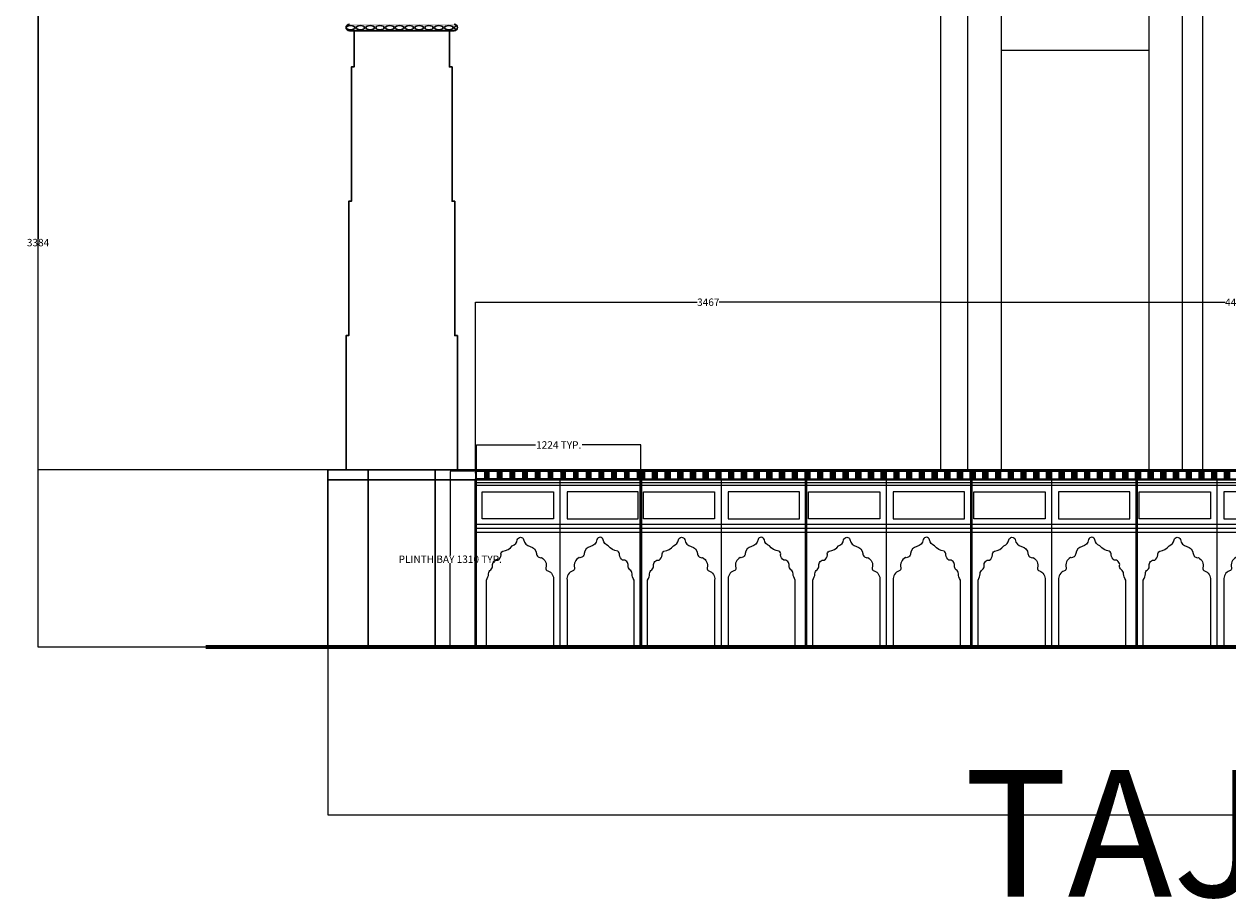
# Model space of a CAD drawing. Units: millimetres. Extents: x 8570 to 49085, y 3782 to 24863.
# Tile 1 of 15: x 8580 to 17549, y 4026 to 10542. Entities that reach past the tile are written whole.
import ezdxf

# ---------------------------------------------------------------- set-up
doc = ezdxf.new("R2010")
doc.units = ezdxf.units.MM
doc.header["$MEASUREMENT"] = 0
doc.header["$PDMODE"] = 3
for name, color, linetype, lineweight in [('A-ANNO-DIMS', 2, 'Continuous', 18), ('A-ANNO-TEXT', 7, 'Continuous', 25), ('A-ELEV-ARCH', 7, 'Continuous', 25), ('A-ELEV-GRND', 7, 'Continuous', 35), ('A-ELEV-MNRT', 7, 'Continuous', 30), ('A-ELEV-PATT', 252, 'Continuous', 13), ('A-ELEV-PIER', 7, 'Continuous', 25), ('A-ELEV-PLIN', 7, 'Continuous', 25)]:
    doc.layers.add(name, color=color, linetype=linetype, lineweight=lineweight)
doc.styles.get("Standard").update_dxf_attribs({"font": 'arial.ttf'})
doc.dimstyles.get("Standard").update_dxf_attribs({"dimtxt": 55, "dimasz": 0.18, "dimexe": 0.18, "dimexo": 0.0625, "dimgap": 0.09, "dimtad": 0, "dimtih": 1, "dimtoh": 1, "dimdec": 0, "dimzin": 0, "dimdsep": 46, "dimtxsty": 'Standard', "dimcen": 0.09, "dimadec": 0, "dimazin": 0, "dimtfac": 1, "dimtdec": 0, "dimtofl": 0, "dimtmove": 0, "dimatfit": 3, "dimfxl": 1, "dimtolj": 1, "dimtzin": 0, "dimarcsym": 0})

# ---------------------------------------------------------------- blocks, each defined once
blk = doc.blocks.new('MINARET-ELEV')
h = blk.add_hatch(color=256)
h.dxf.hatch_style = 1
edge = h.paths.add_edge_path()
edge.add_arc((940, 4615.3), 25, 270, 450, ccw=False)
edge.add_line((940, 4590.3), (160, 4590.3))
edge.add_arc((160, 4615.3), 25, 217.6761, 270, ccw=False)
edge.add_ellipse((127.2, 4613.7), major_axis=(31.8, 0), ratio=0.472441, start_angle=313.43175, end_angle=411.74889)
edge.add_arc((160, 4615.3), 25, 450, 510.08055, ccw=False)
edge.add_line((160, 4640.3), (940, 4640.3))
edge = h.paths.add_edge_path(flags=16)
edge.add_ellipse((347.2, 4613.7), major_axis=(31.8, 0), ratio=0.472441, start_angle=0, end_angle=360, ccw=False)
edge = h.paths.add_edge_path(flags=16)
edge.add_ellipse((420.2, 4613.7), major_axis=(31.8, 0), ratio=0.472441, start_angle=0, end_angle=360, ccw=False)
edge = h.paths.add_edge_path(flags=16)
edge.add_ellipse((274.2, 4613.7), major_axis=(31.8, 0), ratio=0.472441, start_angle=0, end_angle=360, ccw=False)
edge = h.paths.add_edge_path(flags=16)
edge.add_ellipse((493.2, 4613.7), major_axis=(31.8, 0), ratio=0.472441, start_angle=0, end_angle=360, ccw=False)
edge = h.paths.add_edge_path(flags=16)
edge.add_ellipse((198.8, 4613.7), major_axis=(31.8, 0), ratio=0.472441, start_angle=0, end_angle=360, ccw=False)
edge = h.paths.add_edge_path(flags=16)
edge.add_ellipse((566.2, 4613.7), major_axis=(31.8, 0), ratio=0.472441, start_angle=0, end_angle=360, ccw=False)
edge = h.paths.add_edge_path(flags=16)
edge.add_ellipse((639.2, 4613.7), major_axis=(31.8, 0), ratio=0.472441, start_angle=0, end_angle=360, ccw=False)
edge = h.paths.add_edge_path(flags=16)
edge.add_ellipse((712.2, 4613.7), major_axis=(31.8, 0), ratio=0.472441, start_angle=0, end_angle=360, ccw=False)
edge = h.paths.add_edge_path(flags=16)
edge.add_ellipse((785.2, 4613.7), major_axis=(31.8, 0), ratio=0.472441, start_angle=0, end_angle=360, ccw=False)
edge = h.paths.add_edge_path(flags=16)
edge.add_ellipse((858.2, 4613.7), major_axis=(31.8, 0), ratio=0.472441, start_angle=0, end_angle=360, ccw=False)
edge = h.paths.add_edge_path(flags=16)
edge.add_ellipse((931.2, 4613.7), major_axis=(31.8, 0), ratio=0.472441, start_angle=0, end_angle=360, ccw=False)
for p, q in [((160, 4590.3), (940, 4590.3)), ((165, 4590.3), (935, 4590.3)), ((905, 4590.3), (195, 4590.3)), ((300, 0), (300, 1321)), ((800, 0), (800, 1321)), ((1100, 0), (1100, 1321))]:
    blk.add_line(p, q)
for points in [[(135, 1321), (135, 2321), (155, 2321), (155, 3321), (175, 3321), (175, 4321), (195, 4321), (195, 4590.3)], [(965, 1321), (965, 2321), (945, 2321), (945, 3321), (925, 3321), (925, 4321), (905, 4321), (905, 4590.3)], [(0, 1321), (1100, 1321)], [(0, 1246), (1100, 1246)]]:
    blk.add_lwpolyline(points)
for centre, start, end in [((160, 4615.3), 90, 270), ((940, 4615.3), 270, 90)]:
    blk.add_arc(centre, 25, start, end)
at = {"extrusion": (0, 0, -1)}
for centre, start_param, end_param in [((127.2, 4613.7), -1.214257, 1.150222), ((198.8, 4613.7), -6.283185, 0), ((274.2, 4613.7), -6.283185, 0), ((347.2, 4613.7), -6.283185, 0), ((420.2, 4613.7), -6.283185, 0), ((493.2, 4613.7), -6.283185, 0), ((566.2, 4613.7), -6.283185, 0), ((639.2, 4613.7), -6.283185, 0), ((712.2, 4613.7), -6.283185, 0), ((785.2, 4613.7), -6.283185, 0), ((858.2, 4613.7), -6.283185, 0), ((931.2, 4613.7), -6.283185, 0)]:
    blk.add_ellipse(centre, major_axis=(31.8, 0), ratio=0.472441, start_param=start_param, end_param=end_param, dxfattribs=at)
blk = doc.blocks.new('PLINTH-PAIRED-BAY')
for p, q in [((623.5, 0), (623.5, 1246)), ((573.5, 0), (623.5, 0)), ((1173.5, 0), (1223.5, 0))]:
    blk.add_line(p, q)
for points in [[(0, 1309.5), (58.5, 1309.5), (58.5, 1253), (0, 1253)], [(94.7, 1309.5), (153.2, 1309.5), (153.2, 1253), (94.7, 1253)], [(189.5, 1309.5), (248, 1309.5), (248, 1253), (189.5, 1253)], [(284.2, 1309.5), (342.7, 1309.5), (342.7, 1253), (284.2, 1253)], [(378.9, 1309.5), (437.4, 1309.5), (437.4, 1253), (378.9, 1253)], [(473.7, 1309.5), (532.2, 1309.5), (532.2, 1253), (473.7, 1253)], [(568.4, 1309.5), (626.9, 1309.5), (626.9, 1253), (568.4, 1253)], [(663.2, 1309.5), (721.7, 1309.5), (721.7, 1253), (663.2, 1253)], [(757.9, 1309.5), (816.4, 1309.5), (816.4, 1253), (757.9, 1253)], [(852.6, 1309.5), (911.1, 1309.5), (911.1, 1253), (852.6, 1253)], [(947.4, 1309.5), (1005.9, 1309.5), (1005.9, 1253), (947.4, 1253)], [(1042.1, 1309.5), (1100.6, 1309.5), (1100.6, 1253), (1042.1, 1253)], [(1136.8, 1309.5), (1195.3, 1309.5), (1195.3, 1253), (1136.8, 1253)], [(42.5, 1156), (573.5, 1156), (573.5, 956), (42.5, 956)], [(1204.5, 1156), (673.5, 1156), (673.5, 956), (1204.5, 956)]]:
    blk.add_lwpolyline(points, close=True)
for points in [[(573.5, 500), (573.5, 0), (73.5, 0), (73.5, 500, 0.133896), (89, 547, -0.229833), (105, 576, 0.282739), (118.5, 607.5, -0.502693), (159, 648, 0.231145), (182, 687, -0.35399), (196, 714, 0.196071), (266.2, 753.9, 0.282071), (303.4, 799.6, -0.761042), (350.3, 800.8, 0.299945), (398, 749.1, -0.349607), (445.5, 697, 0.443472), (484, 666.5, -0.349941), (517, 591, 0.399043), (530.5, 568, -0.342474)], [(673.5, 500), (673.5, 0), (1173.5, 0), (1173.5, 500, -0.133896), (1158, 547, 0.229833), (1142, 576, -0.282739), (1128.5, 607.5, 0.502693), (1088, 648, -0.231145), (1065, 687, 0.35399), (1051, 714, -0.196071), (980.8, 753.9, -0.282071), (943.6, 799.6, 0.761042), (896.7, 800.8, -0.299945), (849, 749.1, 0.349607), (801.5, 697, -0.443472), (763, 666.5, 0.349941), (730, 591, -0.399043), (716.5, 568, 0.342474)]]:
    blk.add_lwpolyline(points, format="xyb", close=True)
blk = doc.blocks.new('PAVILION-EDGE-PINNACLE')
for p, q in [((10, 8089.5), (160, 8089.5)), ((10, 0), (10, 8069.5)), ((10, 8069.5), (160, 8069.5)), ((160, 0), (160, 8069.5)), ((160, 0), (160, 6876.5)), ((10, 0), (10, 6246.5))]:
    blk.add_line(p, q)
blk.add_lwpolyline([(101.6, 8204.8, 0.216309), (82.9, 8236.3, 0.244698), (64, 8200, 0.244698)], format="xyb")
for centre, radius, start, end in [((153, 8055.1), 147, 117.52778, 166.47476), ((82.6, 8204.4), 19, 193.30654, 1.38797), ((17, 8055.1), 147, 13.52524, 62.47222), ((10, 8079.5), 10, 90, 270), ((160, 8079.5), 10, 270, 90)]:
    blk.add_arc(centre, radius, start, end)
blk = doc.blocks.new('WING-END-PINNACLE')
for p, q in [((10, 8109.5), (210, 8109.5)), ((10, 8089.5), (210, 8089.5)), ((10, 0), (10, 8069.5)), ((10, 8069.5), (210, 8069.5)), ((210, 0), (210, 8069.5))]:
    blk.add_line(p, q)
blk.add_lwpolyline([(127.1, 8207.4, 0.216309), (108.4, 8238.9, 0.244698), (89.5, 8202.5, 0.244698)], format="xyb")
blk.add_circle((110.5, 8181), 7.02)
for centre, radius, start, end in [((-119.7, 8420.4), 336.9, 292.6494, 312.99463), ((108.1, 8206.9), 19, 193.30654, 1.38797), ((340.2, 8421.1), 337.7, 227.0303, 247.32566), ((10, 8099.5), 10, 90, 270), ((10, 8079.5), 10, 90, 270), ((210, 8099.5), 10, 270, 90), ((210, 8079.5), 10, 270, 90)]:
    blk.add_arc(centre, radius, start, end)
blk = doc.blocks.new('WING-TALL-ARCH')
for p, q in [((0, 5946.5), (1100, 5946.5)), ((0, 0), (0, 5946.5)), ((1100, 0), (1100, 5946.5)), ((0, 3123.2), (1100, 3123.2))]:
    blk.add_line(p, q)
for points in [[(47.9, 4748, -0.124525), (550, 5321.3, -0.124525)], [(1052.1, 4748, 0.124525), (550, 5321.3, 0.124525)]]:
    blk.add_lwpolyline(points, format="xyb")
for centre, start, end in [((817.4, 4459.8), 159.46554, 174.14569), ((282.6, 4459.8), 5.85431, 20.53446)]:
    blk.add_arc(centre, 821.7, start, end)
blk = doc.blocks.new('*D17')
at = {"layer": 'A-ANNO-DIMS', "color": 0, "lineweight": -2, "transparency": 16777216}
for p, q in [((11951.4, 7211), (11754.9, 7211)), ((11755.1, 7210.8), (11755.1, 6584.4)), ((11755.1, 5901.7), (11755.1, 6528.1)), ((11951.4, 5901.5), (11754.9, 5901.5))]:
    blk.add_line(p, q, dxfattribs=at)
at = {"layer": 'A-ANNO-DIMS', "color": 0, "transparency": 16777216}
for points in [[(11755, 7210.8), (11755.1, 7210.8), (11755.1, 7211)], [(11755, 5901.7), (11755.1, 5901.7), (11755.1, 5901.5)]]:
    blk.add_solid(points, dxfattribs=at)
at = {"layer": 'Defpoints', "color": 0, "transparency": 16777216}
for p in [(11755.1, 7211), (11951.5, 7211), (11951.5, 5901.5)]:
    blk.add_point(p, dxfattribs=at)
at = {"layer": 'A-ANNO-DIMS', "color": 0, "transparency": 16777216, "insert": (11755.1, 6556.2), "char_height": 55, "attachment_point": 5}
blk.add_mtext('\\A1;PLINTH BAY 1310 TYP.', dxfattribs=at)
blk = doc.blocks.new('*D18')
at = {"layer": 'A-ANNO-DIMS', "color": 0, "lineweight": -2, "transparency": 16777216}
for p, q in [((11951.5, 7211.1), (11951.5, 7407.6)), ((11951.7, 7407.4), (12389.2, 7407.4)), ((13174.8, 7407.4), (12737.3, 7407.4)), ((13175, 7211.1), (13175, 7407.6))]:
    blk.add_line(p, q, dxfattribs=at)
at = {"layer": 'A-ANNO-DIMS', "color": 0, "transparency": 16777216}
for points in [[(11951.7, 7407.5), (11951.7, 7407.4), (11951.5, 7407.4)], [(13174.8, 7407.5), (13174.8, 7407.4), (13175, 7407.4)]]:
    blk.add_solid(points, dxfattribs=at)
at = {"layer": 'Defpoints', "color": 0, "transparency": 16777216}
for p in [(13175, 7407.4), (11951.5, 7211), (13175, 7211)]:
    blk.add_point(p, dxfattribs=at)
at = {"layer": 'A-ANNO-DIMS', "color": 0, "transparency": 16777216, "insert": (12563.2, 7407.4), "char_height": 55, "attachment_point": 5}
blk.add_mtext('\\A1;1224 TYP.', dxfattribs=at)
blk = doc.blocks.new('*D43')
at = {"layer": 'A-ANNO-DIMS', "color": 0, "lineweight": -2, "transparency": 16777216}
for p, q in [((10844, 5901.4), (10844, 4653.3)), ((33971, 5901.4), (33971, 4653.3)), ((10844.2, 4653.5), (22303.5, 4653.5)), ((33970.8, 4653.5), (22511.5, 4653.5))]:
    blk.add_line(p, q, dxfattribs=at)
at = {"layer": 'A-ANNO-DIMS', "color": 0, "transparency": 16777216}
for points in [[(10844.2, 4653.5), (10844.2, 4653.5), (10844, 4653.5)], [(33970.8, 4653.5), (33970.8, 4653.5), (33971, 4653.5)]]:
    blk.add_solid(points, dxfattribs=at)
at = {"layer": 'Defpoints', "color": 0, "transparency": 16777216}
for p in [(10844, 5901.5), (33971, 5901.5), (33971, 4653.5)]:
    blk.add_point(p, dxfattribs=at)
at = {"layer": 'A-ANNO-DIMS', "color": 0, "transparency": 16777216, "insert": (22407.5, 4653.5), "char_height": 55, "attachment_point": 5}
blk.add_mtext('\\A1;23127', dxfattribs=at)
blk = doc.blocks.new('*D44')
at = {"layer": 'A-ANNO-DIMS', "color": 0, "lineweight": -2, "transparency": 16777216}
for p, q in [((22399.7, 24863), (8684.3, 24863)), ((8684.5, 24862.8), (8684.5, 15410.4)), ((8684.5, 5901.7), (8684.5, 15354.1)), ((10843.9, 5901.5), (8684.3, 5901.5))]:
    blk.add_line(p, q, dxfattribs=at)
at = {"layer": 'A-ANNO-DIMS', "color": 0, "transparency": 16777216}
for points in [[(8684.5, 24862.8), (8684.5, 24862.8), (8684.5, 24863)], [(8684.5, 5901.7), (8684.5, 5901.7), (8684.5, 5901.5)]]:
    blk.add_solid(points, dxfattribs=at)
at = {"layer": 'Defpoints', "color": 0, "transparency": 16777216}
for p in [(8684.5, 24863), (22399.8, 24863), (10844, 5901.5)]:
    blk.add_point(p, dxfattribs=at)
at = {"layer": 'A-ANNO-DIMS', "color": 0, "transparency": 16777216, "insert": (8684.5, 15382.2), "char_height": 55, "attachment_point": 5}
blk.add_mtext('\\A1;18961', dxfattribs=at)
blk = doc.blocks.new('*D45')
at = {"layer": 'A-ANNO-DIMS', "color": 0, "lineweight": -2, "transparency": 16777216}
for p, q in [((11944, 7222.6), (11944, 8470.7)), ((11944.2, 8470.5), (13595.3, 8470.5)), ((15410.8, 8470.5), (13759.7, 8470.5)), ((15411, 7222.6), (15411, 8470.7))]:
    blk.add_line(p, q, dxfattribs=at)
at = {"layer": 'A-ANNO-DIMS', "color": 0, "transparency": 16777216}
for points in [[(11944.2, 8470.5), (11944.2, 8470.5), (11944, 8470.5)], [(15410.8, 8470.5), (15410.8, 8470.5), (15411, 8470.5)]]:
    blk.add_solid(points, dxfattribs=at)
at = {"layer": 'Defpoints', "color": 0, "transparency": 16777216}
for p in [(15411, 8470.5), (11944, 7222.5), (15411, 7222.5)]:
    blk.add_point(p, dxfattribs=at)
at = {"layer": 'A-ANNO-DIMS', "color": 0, "transparency": 16777216, "insert": (13677.5, 8470.5), "char_height": 55, "attachment_point": 5}
blk.add_mtext('\\A1;3467', dxfattribs=at)
blk = doc.blocks.new('*D46')
at = {"layer": 'A-ANNO-DIMS', "color": 0, "lineweight": -2, "transparency": 16777216}
for p, q in [((15411, 7222.6), (15411, 8470.7)), ((15411.2, 8470.5), (17527.8, 8470.5)), ((19810.8, 8470.5), (17694.2, 8470.5)), ((19811, 7222.6), (19811, 8470.7))]:
    blk.add_line(p, q, dxfattribs=at)
at = {"layer": 'A-ANNO-DIMS', "color": 0, "transparency": 16777216}
for points in [[(15411.2, 8470.5), (15411.2, 8470.5), (15411, 8470.5)], [(19810.8, 8470.5), (19810.8, 8470.5), (19811, 8470.5)]]:
    blk.add_solid(points, dxfattribs=at)
at = {"layer": 'Defpoints', "color": 0, "transparency": 16777216}
for p in [(19811, 8470.5), (15411, 7222.5), (19811, 7222.5)]:
    blk.add_point(p, dxfattribs=at)
at = {"layer": 'A-ANNO-DIMS', "color": 0, "transparency": 16777216, "insert": (17611, 8470.5), "char_height": 55, "attachment_point": 5}
blk.add_mtext('\\A1;4400', dxfattribs=at)
blk = doc.blocks.new('*D59')
at = {"layer": 'A-ANNO-DIMS', "color": 0, "lineweight": -2, "transparency": 16777216}
for p, q in [((32990.4, 10606.5), (8684.3, 10606.5)), ((8684.5, 10606.3), (8684.5, 8942.7)), ((8684.5, 7222.7), (8684.5, 8886.3)), ((32870.9, 7222.5), (8684.3, 7222.5))]:
    blk.add_line(p, q, dxfattribs=at)
at = {"layer": 'A-ANNO-DIMS', "color": 0, "transparency": 16777216}
for points in [[(8684.5, 10606.3), (8684.5, 10606.3), (8684.5, 10606.5)], [(8684.5, 7222.7), (8684.5, 7222.7), (8684.5, 7222.5)]]:
    blk.add_solid(points, dxfattribs=at)
at = {"layer": 'Defpoints', "color": 0, "transparency": 16777216}
for p in [(8684.5, 10606.5), (32990.5, 10606.5), (32871, 7222.5)]:
    blk.add_point(p, dxfattribs=at)
at = {"layer": 'A-ANNO-DIMS', "color": 0, "transparency": 16777216, "insert": (8684.5, 8914.5), "char_height": 55, "attachment_point": 5}
blk.add_mtext('\\A1;3384', dxfattribs=at)

msp = doc.modelspace()

# ---------------------------------------------------------------- hatches: boundary and pattern name
at = {"layer": 'A-ELEV-PATT'}
h = msp.add_hatch(dxfattribs=at)
h.set_pattern_fill('ANSI31', color=256)
h.paths.add_polyline_path([(11944, 7222.5), (11944, 7147.5), (13175, 7147.5), (13175, 7222.5)])
h.paths.add_polyline_path([(12862.63, 7211), (12862.63, 7154.5), (12804.13, 7154.5), (12804.13, 7211)], flags=16)
h.paths.add_polyline_path([(12898.87, 7211), (12957.37, 7211), (12957.37, 7154.5), (12898.87, 7154.5)], flags=16)
h.paths.add_polyline_path([(12767.89, 7211), (12767.89, 7154.5), (12709.39, 7154.5), (12709.39, 7211)], flags=16)
h.paths.add_polyline_path([(12993.61, 7211), (13052.11, 7211), (13052.11, 7154.5), (12993.61, 7154.5)], flags=16)
h.paths.add_polyline_path([(12673.16, 7211), (12673.16, 7154.5), (12614.66, 7154.5), (12614.66, 7211)], flags=16)
h.paths.add_polyline_path([(13088.34, 7211), (13146.84, 7211), (13146.84, 7154.5), (13088.34, 7154.5)], flags=16)
h.paths.add_polyline_path([(12578.42, 7211), (12578.42, 7154.5), (12519.92, 7154.5), (12519.92, 7211)], flags=16)
h.paths.add_polyline_path([(12483.68, 7211), (12483.68, 7154.5), (12425.18, 7154.5), (12425.18, 7211)], flags=16)
h.paths.add_polyline_path([(12388.95, 7211), (12388.95, 7154.5), (12330.45, 7154.5), (12330.45, 7211)], flags=16)
h.paths.add_polyline_path([(12294.21, 7211), (12294.21, 7154.5), (12235.71, 7154.5), (12235.71, 7211)], flags=16)
h.paths.add_polyline_path([(12199.47, 7211), (12199.47, 7154.5), (12140.97, 7154.5), (12140.97, 7211)], flags=16)
h.paths.add_polyline_path([(12104.74, 7211), (12104.74, 7154.5), (12046.24, 7154.5), (12046.24, 7211)], flags=16)
h.paths.add_polyline_path([(12010, 7211), (12010, 7154.5), (11951.5, 7154.5), (11951.5, 7211)], flags=16)
h = msp.add_hatch(dxfattribs=at)
h.set_pattern_fill('ANSI31', color=256)
h.paths.add_polyline_path([(13175, 7222.5), (14406, 7222.5), (14406, 7147.5), (13175, 7147.5)])
h.paths.add_polyline_path([(13487.37, 7154.5), (13545.87, 7154.5), (13545.87, 7211), (13487.37, 7211)], flags=16)
h.paths.add_polyline_path([(13451.13, 7211), (13392.63, 7211), (13392.63, 7154.5), (13451.13, 7154.5)], flags=16)
h.paths.add_polyline_path([(13582.11, 7154.5), (13640.61, 7154.5), (13640.61, 7211), (13582.11, 7211)], flags=16)
h.paths.add_polyline_path([(13356.39, 7211), (13297.89, 7211), (13297.89, 7154.5), (13356.39, 7154.5)], flags=16)
h.paths.add_polyline_path([(13676.84, 7154.5), (13735.34, 7154.5), (13735.34, 7211), (13676.84, 7211)], flags=16)
h.paths.add_polyline_path([(13261.66, 7211), (13203.16, 7211), (13203.16, 7154.5), (13261.66, 7154.5)], flags=16)
h.paths.add_polyline_path([(13771.58, 7154.5), (13830.08, 7154.5), (13830.08, 7211), (13771.58, 7211)], flags=16)
h.paths.add_polyline_path([(13866.32, 7154.5), (13924.82, 7154.5), (13924.82, 7211), (13866.32, 7211)], flags=16)
h.paths.add_polyline_path([(13961.05, 7154.5), (14019.55, 7154.5), (14019.55, 7211), (13961.05, 7211)], flags=16)
h.paths.add_polyline_path([(14055.79, 7154.5), (14114.29, 7154.5), (14114.29, 7211), (14055.79, 7211)], flags=16)
h.paths.add_polyline_path([(14150.53, 7154.5), (14209.03, 7154.5), (14209.03, 7211), (14150.53, 7211)], flags=16)
h.paths.add_polyline_path([(14245.26, 7154.5), (14303.76, 7154.5), (14303.76, 7211), (14245.26, 7211)], flags=16)
h.paths.add_polyline_path([(14340, 7154.5), (14398.5, 7154.5), (14398.5, 7211), (14340, 7211)], flags=16)
h = msp.add_hatch(dxfattribs=at)
h.set_pattern_fill('ANSI31', color=256)
h.set_pattern_definition([(45, (1231, 0), (-0.0883883476, 0.0883883476), [])])
h.paths.add_polyline_path([(14406, 7222.5), (15637, 7222.5), (15637, 7147.5), (14406, 7147.5)])
h.paths.add_polyline_path([(14718.37, 7154.5), (14776.87, 7154.5), (14776.87, 7211), (14718.37, 7211)], flags=16)
h.paths.add_polyline_path([(14682.13, 7211), (14623.63, 7211), (14623.63, 7154.5), (14682.13, 7154.5)], flags=16)
h.paths.add_polyline_path([(14813.11, 7154.5), (14871.61, 7154.5), (14871.61, 7211), (14813.11, 7211)], flags=16)
h.paths.add_polyline_path([(14587.39, 7211), (14528.89, 7211), (14528.89, 7154.5), (14587.39, 7154.5)], flags=16)
h.paths.add_polyline_path([(14907.84, 7154.5), (14966.34, 7154.5), (14966.34, 7211), (14907.84, 7211)], flags=16)
h.paths.add_polyline_path([(14492.66, 7211), (14434.16, 7211), (14434.16, 7154.5), (14492.66, 7154.5)], flags=16)
h.paths.add_polyline_path([(15002.58, 7154.5), (15061.08, 7154.5), (15061.08, 7211), (15002.58, 7211)], flags=16)
h.paths.add_polyline_path([(15097.32, 7154.5), (15155.82, 7154.5), (15155.82, 7211), (15097.32, 7211)], flags=16)
h.paths.add_polyline_path([(15192.05, 7154.5), (15250.55, 7154.5), (15250.55, 7211), (15192.05, 7211)], flags=16)
h.paths.add_polyline_path([(15286.79, 7154.5), (15345.29, 7154.5), (15345.29, 7211), (15286.79, 7211)], flags=16)
h.paths.add_polyline_path([(15381.53, 7154.5), (15440.03, 7154.5), (15440.03, 7211), (15381.53, 7211)], flags=16)
h.paths.add_polyline_path([(15476.26, 7154.5), (15534.76, 7154.5), (15534.76, 7211), (15476.26, 7211)], flags=16)
h.paths.add_polyline_path([(15571, 7154.5), (15629.5, 7154.5), (15629.5, 7211), (15571, 7211)], flags=16)
h = msp.add_hatch(dxfattribs=at)
h.set_pattern_fill('ANSI31', color=256)
h.set_pattern_definition([(45, (2462, 0), (-0.0883883476, 0.0883883476), [])])
h.paths.add_polyline_path([(15637, 7222.5), (16868, 7222.5), (16868, 7147.5), (15637, 7147.5)])
h.paths.add_polyline_path([(15949.37, 7154.5), (16007.87, 7154.5), (16007.87, 7211), (15949.37, 7211)], flags=16)
h.paths.add_polyline_path([(15913.13, 7211), (15854.63, 7211), (15854.63, 7154.5), (15913.13, 7154.5)], flags=16)
h.paths.add_polyline_path([(16044.11, 7154.5), (16102.61, 7154.5), (16102.61, 7211), (16044.11, 7211)], flags=16)
h.paths.add_polyline_path([(15818.39, 7211), (15759.89, 7211), (15759.89, 7154.5), (15818.39, 7154.5)], flags=16)
h.paths.add_polyline_path([(16138.84, 7154.5), (16197.34, 7154.5), (16197.34, 7211), (16138.84, 7211)], flags=16)
h.paths.add_polyline_path([(15723.66, 7211), (15665.16, 7211), (15665.16, 7154.5), (15723.66, 7154.5)], flags=16)
h.paths.add_polyline_path([(16233.58, 7154.5), (16292.08, 7154.5), (16292.08, 7211), (16233.58, 7211)], flags=16)
h.paths.add_polyline_path([(16328.32, 7154.5), (16386.82, 7154.5), (16386.82, 7211), (16328.32, 7211)], flags=16)
h.paths.add_polyline_path([(16423.05, 7154.5), (16481.55, 7154.5), (16481.55, 7211), (16423.05, 7211)], flags=16)
h.paths.add_polyline_path([(16517.79, 7154.5), (16576.29, 7154.5), (16576.29, 7211), (16517.79, 7211)], flags=16)
h.paths.add_polyline_path([(16612.53, 7154.5), (16671.03, 7154.5), (16671.03, 7211), (16612.53, 7211)], flags=16)
h.paths.add_polyline_path([(16707.26, 7154.5), (16765.76, 7154.5), (16765.76, 7211), (16707.26, 7211)], flags=16)
h.paths.add_polyline_path([(16802, 7154.5), (16860.5, 7154.5), (16860.5, 7211), (16802, 7211)], flags=16)
h = msp.add_hatch(dxfattribs=at)
h.set_pattern_fill('ANSI31', color=256)
h.set_pattern_definition([(45, (3693, 0), (-0.0883883476, 0.0883883476), [])])
h.paths.add_polyline_path([(16868, 7222.5), (18099, 7222.5), (18099, 7147.5), (16868, 7147.5)])
h.paths.add_polyline_path([(17180.37, 7154.5), (17238.87, 7154.5), (17238.87, 7211), (17180.37, 7211)], flags=16)
h.paths.add_polyline_path([(17144.13, 7211), (17085.63, 7211), (17085.63, 7154.5), (17144.13, 7154.5)], flags=16)
h.paths.add_polyline_path([(17275.11, 7154.5), (17333.61, 7154.5), (17333.61, 7211), (17275.11, 7211)], flags=16)
h.paths.add_polyline_path([(17049.39, 7211), (16990.89, 7211), (16990.89, 7154.5), (17049.39, 7154.5)], flags=16)
h.paths.add_polyline_path([(17369.84, 7154.5), (17428.34, 7154.5), (17428.34, 7211), (17369.84, 7211)], flags=16)
h.paths.add_polyline_path([(16954.66, 7211), (16896.16, 7211), (16896.16, 7154.5), (16954.66, 7154.5)], flags=16)
h.paths.add_polyline_path([(17464.58, 7154.5), (17523.08, 7154.5), (17523.08, 7211), (17464.58, 7211)], flags=16)
h.paths.add_polyline_path([(17559.32, 7154.5), (17617.82, 7154.5), (17617.82, 7211), (17559.32, 7211)], flags=16)
h.paths.add_polyline_path([(17654.05, 7154.5), (17712.55, 7154.5), (17712.55, 7211), (17654.05, 7211)], flags=16)
h.paths.add_polyline_path([(17748.79, 7154.5), (17807.29, 7154.5), (17807.29, 7211), (17748.79, 7211)], flags=16)
h.paths.add_polyline_path([(17843.53, 7154.5), (17902.03, 7154.5), (17902.03, 7211), (17843.53, 7211)], flags=16)
h.paths.add_polyline_path([(17938.26, 7154.5), (17996.76, 7154.5), (17996.76, 7211), (17938.26, 7211)], flags=16)
h.paths.add_polyline_path([(18033, 7154.5), (18091.5, 7154.5), (18091.5, 7211), (18033, 7211)], flags=16)

# ---------------------------------------------------------------- linework, layer by layer
at = {"layer": 'A-ELEV-GRND', "const_width": 30}
msp.add_lwpolyline([(9932.5, 5901.52), (34807, 5902)], dxfattribs=at)
at = {"layer": 'A-ELEV-PLIN'}
for p, q in [((14406, 5901.5), (14406, 7222.5)), ((15637, 5901.5), (15637, 7222.5)), ((16868, 5901.5), (16868, 7222.5))]:
    msp.add_line(p, q, dxfattribs=at)
for points in [[(11944, 7222.5), (21944, 7222.5)], [(11944, 7147.5), (21944, 7147.5)], [(11944, 7127.5), (32871, 7127.5)], [(11944, 7107.5), (32871, 7107.5)], [(11944, 6817.5), (32871, 6817.5)], [(11944, 6787.5), (32871, 6787.5)], [(11944, 6757.5), (32871, 6757.5)]]:
    msp.add_lwpolyline(points, dxfattribs=at)
at = {"layer": 'A-ELEV-PLIN', "const_width": 20}
for points in [[(13175, 5901.5), (13175, 7222.5)], [(14406, 5901.5), (14406, 7222.5)], [(15637, 5901.5), (15637, 7222.5)], [(16868, 5901.5), (16868, 7222.5)], [(11944, 7147.5), (11944.03, 5901.55)]]:
    msp.add_lwpolyline(points, dxfattribs=at)

# ---------------------------------------------------------------- block references
at = {"layer": 'A-ELEV-ARCH', "extrusion": (0, 0, -1), "zscale": -1}
msp.add_blockref('WING-TALL-ARCH', (-16961, 7222.5), dxfattribs=at)
at = {"layer": 'A-ELEV-MNRT', "extrusion": (0, 0, -1), "zscale": -1}
msp.add_blockref('MINARET-ELEV', (-11944, 5901.5), dxfattribs=at)
at = {"layer": 'A-ELEV-PIER', "extrusion": (0, 0, -1), "zscale": -1}
for name, p in [('WING-END-PINNACLE', (-15621, 7222.5)), ('PAVILION-EDGE-PINNACLE', (-17371, 7222.5))]:
    msp.add_blockref(name, p, dxfattribs=at)
at = {"layer": 'A-ELEV-PLIN'}
msp.add_blockref('PLINTH-PAIRED-BAY', (11951.5, 5901.5), dxfattribs=at)
at = {"layer": 'A-ELEV-PLIN', "extrusion": (0, 0, -1), "zscale": -1}
for p in [(-14398.5, 5901.5), (-15629.5, 5901.5), (-16860.5, 5901.5), (-18091.5, 5901.5)]:
    msp.add_blockref('PLINTH-PAIRED-BAY', p, dxfattribs=at)

# ---------------------------------------------------------------- texts
at = {"layer": 'A-ANNO-TEXT'}
msp.add_text('TAJ MAHAL ELEVATION', height=943, dxfattribs=at).set_placement((15583.5, 4043))

# ---------------------------------------------------------------- dimensions: what is measured, and where the dimension line sits
at = {"layer": 'A-ANNO-DIMS'}
for base, p1, p2, angle, picture, middle in [((8684.5, 24862.95), (10844, 5901.5), (22399.75, 24862.95), 90, '*D44', (8684.5, 15382.23)), ((8684.5, 10606.5), (32871, 7222.5), (32990.5, 10606.5), 90, '*D59', (8684.5, 8914.5)), ((19811, 8470.5), (15411, 7222.5), (19811, 7222.5), 0, '*D46', (17611, 8470.5))]:
    dim = msp.add_linear_dim(base=base, p1=p1, p2=p2, angle=angle, dimstyle='Standard', override={"dimdec": 0, "dimlfac": 1, "dimrnd": 0, "dimzin": 0, "dimdsep": 46, "dimlunit": 2}, dxfattribs=at)
    dim.commit()
    dim.dimension.update_dxf_attribs({"geometry": picture, "text_midpoint": middle})
for base, p1, p2, picture, middle in [((15411, 8470.5), (11944, 7222.5), (15411, 7222.5), '*D45', (13677.5, 8470.5)), ((33971, 4653.5), (10844, 5901.5), (33971, 5901.5), '*D43', (22407.5, 4653.5))]:
    dim = msp.add_linear_dim(base=base, p1=p1, p2=p2, dimstyle='Standard', override={"dimdec": 0, "dimlfac": 1, "dimrnd": 0, "dimzin": 0, "dimdsep": 46, "dimlunit": 2}, dxfattribs=at)
    dim.commit()
    dim.dimension.update_dxf_attribs({"geometry": picture, "text_midpoint": middle})
dim = msp.add_linear_dim(base=(13175, 7407.425), p1=(11951.5, 7211), p2=(13175, 7211), text='<> TYP.', dimstyle='Standard', override={"dimdec": 0, "dimlfac": 1, "dimrnd": 0, "dimzin": 0, "dimdsep": 46, "dimlunit": 2}, dxfattribs=at)
dim.commit()
dim.dimension.update_dxf_attribs({"geometry": '*D18', "text_midpoint": (12563.25, 7407.425)})
dim = msp.add_linear_dim(base=(11755.075, 7211), p1=(11951.5, 5901.5), p2=(11951.5, 7211), angle=90, text='PLINTH BAY <> TYP.', dimstyle='Standard', override={"dimdec": 0, "dimlfac": 1, "dimrnd": 0, "dimzin": 0, "dimdsep": 46, "dimlunit": 2}, dxfattribs=at)
dim.commit()
dim.dimension.update_dxf_attribs({"geometry": '*D17', "text_midpoint": (11755.075, 6556.25)})

doc.saveas('drawing.dxf')
